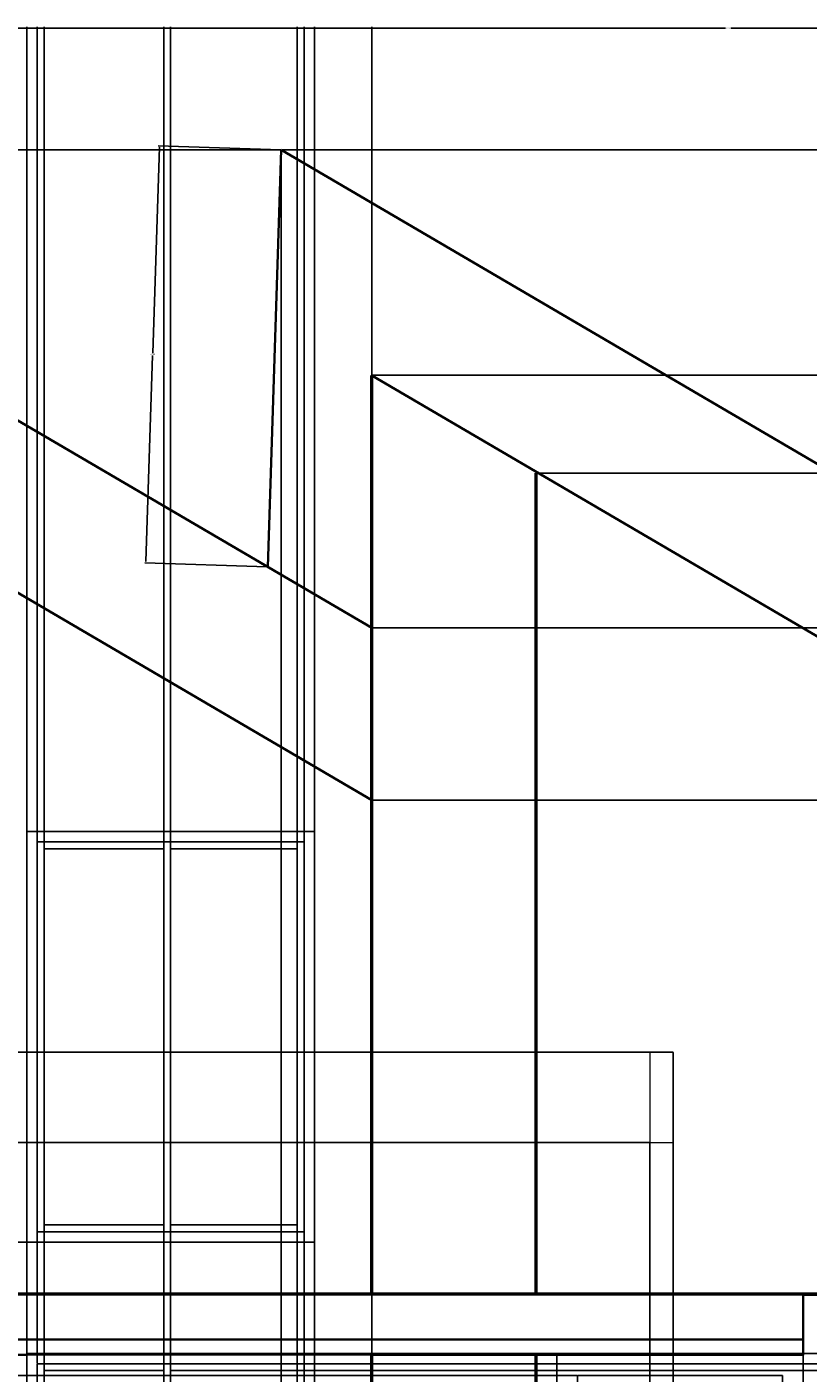
# Model space of a CAD drawing. Units: inches. Extents: x 27 to 409, y -26 to 294.
# Tile 4 of 7: x 116 to 230, y 97 to 294. Entities that reach past the tile are written whole.
import ezdxf

# ---------------------------------------------------------------- set-up
doc = ezdxf.new("R2010")
doc.units = ezdxf.units.IN
doc.header["$MEASUREMENT"] = 0
for name, color, linetype, lineweight in [('A-ANNO-DIMS', 2, 'Continuous', 18), ('A-DOOR', 3, 'Continuous', 25), ('A-ELEV', 8, 'Continuous', 18), ('A-GLAZ', 4, 'Continuous', 25), ('A-ROOF', 1, 'Continuous', 35), ('A-WALL', 7, 'Continuous', 50)]:
    doc.layers.add(name, color=color, linetype=linetype, lineweight=lineweight)
doc.styles.get("Standard").update_dxf_attribs({"font": 'arial.ttf'})
doc.dimstyles.get("Standard").update_dxf_attribs({"dimtxt": 0.18, "dimasz": 0.18, "dimexe": 0.18, "dimexo": 0.0625, "dimgap": 0.09, "dimtad": 0, "dimtih": 1, "dimtoh": 1, "dimdec": 4, "dimzin": 0, "dimdsep": 46, "dimtxsty": 'Standard', "dimcen": 0.09, "dimadec": 0, "dimazin": 0, "dimtfac": 1, "dimtdec": 4, "dimtofl": 0, "dimtmove": 0, "dimatfit": 3, "dimfxl": 1, "dimtolj": 1, "dimtzin": 0, "dimarcsym": 0})

# ---------------------------------------------------------------- blocks, each defined once
blk = doc.blocks.new('*U2')
for p, q in [((1.5, 1.5), (1.5, 58.5)), ((1.5, 58.5), (21, 58.5)), ((21, 1.5), (21, 58.5)), ((21, 58.5), (40.5, 58.5)), ((40.5, 58.5), (40.5, 1.5)), ((21, 1.5), (1.5, 1.5)), ((40.5, 1.5), (21, 1.5))]:
    blk.add_line(p, q)
blk.add_lwpolyline([(0, 0), (0, 60), (42, 60), (42, 0)], close=True)
for points in [[(20, 57.5), (20, 2.5), (2.5, 2.5), (2.5, 57.5), (20, 57.5)], [(21, 57.5), (39.5, 57.5), (39.5, 2.5), (21, 2.5)]]:
    blk.add_lwpolyline(points)
blk = doc.blocks.new('*U5')
blk.add_lwpolyline([(3.12, 0.01), (0.12, 0.01), (0.12, 84.01), (36.12, 84.01), (36.12, 0.01), (33.12, 0.01)])
for points in [[(33.12, 80.99), (33.12, 0.01), (3.12, 0.01), (3.12, 80.99)], [(29.12, 6.01), (29.12, 74.99), (7.12, 74.99), (7.12, 6.01)]]:
    blk.add_lwpolyline(points, close=True)
blk.add_circle((31.12, 42.01), 1)
blk = doc.blocks.new('*D7')
at = {"layer": 'A-ANNO-DIMS', "color": 0, "lineweight": -2, "transparency": 16777216}
for p, q in [((45.58, 108.44), (45.58, 293.63)), ((45.76, 293.45), (217.77, 293.45)), ((390.53, 293.45), (218.52, 293.45)), ((390.71, 136.32), (390.71, 293.63))]:
    blk.add_line(p, q, dxfattribs=at)
at = {"layer": 'A-ANNO-DIMS', "color": 0, "transparency": 16777216}
for points in [[(45.76, 293.48), (45.76, 293.42), (45.58, 293.45)], [(390.53, 293.48), (390.53, 293.42), (390.71, 293.45)]]:
    blk.add_solid(points, dxfattribs=at)
at = {"layer": 'Defpoints', "color": 0, "transparency": 16777216}
for p in [(390.71, 293.45), (390.71, 136.26), (45.58, 108.38)]:
    blk.add_point(p, dxfattribs=at)
at = {"layer": 'A-ANNO-DIMS', "color": 0, "transparency": 16777216, "insert": (218.14, 293.45), "char_height": 0.18, "attachment_point": 5}
blk.add_mtext('\\A1;345.1', dxfattribs=at)
blk = doc.blocks.new('*D15')
at = {"layer": 'A-ANNO-DIMS', "color": 0, "lineweight": -2, "transparency": 16777216}
for p, q in [((152.83, 275.59), (152.83, -26.5)), ((115.67, 115.93), (115.67, -26.5)), ((115.85, -26.32), (133.86, -26.32)), ((152.65, -26.32), (134.64, -26.32))]:
    blk.add_line(p, q, dxfattribs=at)
at = {"layer": 'A-ANNO-DIMS', "color": 0, "transparency": 16777216}
for points in [[(115.85, -26.29), (115.85, -26.35), (115.67, -26.32)], [(152.65, -26.29), (152.65, -26.35), (152.83, -26.32)]]:
    blk.add_solid(points, dxfattribs=at)
at = {"layer": 'Defpoints', "color": 0, "transparency": 16777216}
for p in [(152.83, 275.65), (115.67, 116), (152.83, -26.32)]:
    blk.add_point(p, dxfattribs=at)
at = {"layer": 'A-ANNO-DIMS', "color": 0, "transparency": 16777216, "insert": (134.25, -26.32), "char_height": 0.18, "attachment_point": 5}
blk.add_mtext('\\A1;37.17', dxfattribs=at)
blk = doc.blocks.new('*D16')
at = {"layer": 'A-ANNO-DIMS', "color": 0, "lineweight": -2, "transparency": 16777216}
for p, q in [((152.83, 275.59), (152.83, -26.5)), ((166.08, 180.52), (166.08, -26.5)), ((153.01, -26.32), (159, -26.32)), ((165.9, -26.32), (159.91, -26.32))]:
    blk.add_line(p, q, dxfattribs=at)
at = {"layer": 'A-ANNO-DIMS', "color": 0, "transparency": 16777216}
for points in [[(153.01, -26.29), (153.01, -26.35), (152.83, -26.32)], [(165.9, -26.29), (165.9, -26.35), (166.08, -26.32)]]:
    blk.add_solid(points, dxfattribs=at)
at = {"layer": 'Defpoints', "color": 0, "transparency": 16777216}
for p in [(152.83, 275.65), (166.08, 180.59), (166.08, -26.32)]:
    blk.add_point(p, dxfattribs=at)
at = {"layer": 'A-ANNO-DIMS', "color": 0, "transparency": 16777216, "insert": (159.45, -26.32), "char_height": 0.18, "attachment_point": 5}
blk.add_mtext('\\A1;13.242', dxfattribs=at)
blk = doc.blocks.new('*D17')
at = {"layer": 'A-ANNO-DIMS', "color": 0, "lineweight": -2, "transparency": 16777216}
for p, q in [((166.08, 180.52), (166.08, -26.5)), ((187.49, -8.58), (187.49, -26.5)), ((166.26, -26.32), (176.39, -26.32)), ((187.31, -26.32), (177.18, -26.32))]:
    blk.add_line(p, q, dxfattribs=at)
at = {"layer": 'A-ANNO-DIMS', "color": 0, "transparency": 16777216}
for points in [[(166.26, -26.29), (166.26, -26.35), (166.08, -26.32)], [(187.31, -26.29), (187.31, -26.35), (187.49, -26.32)]]:
    blk.add_solid(points, dxfattribs=at)
at = {"layer": 'Defpoints', "color": 0, "transparency": 16777216}
for p in [(166.08, 180.59), (187.49, -8.52), (187.49, -26.32)]:
    blk.add_point(p, dxfattribs=at)
at = {"layer": 'A-ANNO-DIMS', "color": 0, "transparency": 16777216, "insert": (176.78, -26.32), "char_height": 0.18, "attachment_point": 5}
blk.add_mtext('\\A1;21.42', dxfattribs=at)
blk = doc.blocks.new('*D18')
at = {"layer": 'A-ANNO-DIMS', "color": 0, "lineweight": -2, "transparency": 16777216}
for p, q in [((206.7, 130.47), (206.7, -26.5)), ((187.49, -8.58), (187.49, -26.5)), ((187.67, -26.32), (196.64, -26.32)), ((206.52, -26.32), (197.55, -26.32))]:
    blk.add_line(p, q, dxfattribs=at)
at = {"layer": 'A-ANNO-DIMS', "color": 0, "transparency": 16777216}
for points in [[(187.67, -26.29), (187.67, -26.35), (187.49, -26.32)], [(206.52, -26.29), (206.52, -26.35), (206.7, -26.32)]]:
    blk.add_solid(points, dxfattribs=at)
at = {"layer": 'Defpoints', "color": 0, "transparency": 16777216}
for p in [(206.7, 130.53), (187.49, -8.52), (206.7, -26.32)]:
    blk.add_point(p, dxfattribs=at)
at = {"layer": 'A-ANNO-DIMS', "color": 0, "transparency": 16777216, "insert": (197.09, -26.32), "char_height": 0.18, "attachment_point": 5}
blk.add_mtext('\\A1;19.203', dxfattribs=at)
blk = doc.blocks.new('*D19')
at = {"layer": 'A-ANNO-DIMS', "color": 0, "lineweight": -2, "transparency": 16777216}
for p, q in [((210.09, 143.71), (210.09, -26.5)), ((206.7, 130.47), (206.7, -26.5)), ((206.88, -26.32), (208, -26.32)), ((209.91, -26.32), (208.79, -26.32))]:
    blk.add_line(p, q, dxfattribs=at)
at = {"layer": 'A-ANNO-DIMS', "color": 0, "transparency": 16777216}
for points in [[(206.88, -26.29), (206.88, -26.35), (206.7, -26.32)], [(209.91, -26.29), (209.91, -26.35), (210.09, -26.32)]]:
    blk.add_solid(points, dxfattribs=at)
at = {"layer": 'Defpoints', "color": 0, "transparency": 16777216}
for p in [(210.09, 143.77), (206.7, 130.53), (210.09, -26.32)]:
    blk.add_point(p, dxfattribs=at)
at = {"layer": 'A-ANNO-DIMS', "color": 0, "transparency": 16777216, "insert": (208.39, -26.32), "char_height": 0.18, "attachment_point": 5}
blk.add_mtext('\\A1;3.394', dxfattribs=at)
blk = doc.blocks.new('*D20')
at = {"layer": 'A-ANNO-DIMS', "color": 0, "lineweight": -2, "transparency": 16777216}
for p, q in [((210.09, 143.71), (210.09, -26.5)), ((230.52, -8.58), (230.52, -26.5)), ((210.27, -26.32), (219.84, -26.32)), ((230.34, -26.32), (220.77, -26.32))]:
    blk.add_line(p, q, dxfattribs=at)
at = {"layer": 'A-ANNO-DIMS', "color": 0, "transparency": 16777216}
for points in [[(210.27, -26.29), (210.27, -26.35), (210.09, -26.32)], [(230.34, -26.29), (230.34, -26.35), (230.52, -26.32)]]:
    blk.add_solid(points, dxfattribs=at)
at = {"layer": 'Defpoints', "color": 0, "transparency": 16777216}
for p in [(210.09, 143.77), (230.52, -8.52), (230.52, -26.32)]:
    blk.add_point(p, dxfattribs=at)
at = {"layer": 'A-ANNO-DIMS', "color": 0, "transparency": 16777216, "insert": (220.31, -26.32), "char_height": 0.18, "attachment_point": 5}
blk.add_mtext('\\A1;20.435', dxfattribs=at)
blk = doc.blocks.new('*D30')
at = {"layer": 'A-ANNO-DIMS', "color": 0, "lineweight": -2, "transparency": 16777216}
for p, q in [((206.63, 130.53), (27.6, 130.53)), ((27.78, 130.35), (27.78, 123.45)), ((27.78, 116.18), (27.78, 123.08)), ((115.6, 116), (27.6, 116))]:
    blk.add_line(p, q, dxfattribs=at)
at = {"layer": 'A-ANNO-DIMS', "color": 0, "transparency": 16777216}
for points in [[(27.75, 130.35), (27.81, 130.35), (27.78, 130.53)], [(27.75, 116.18), (27.81, 116.18), (27.78, 116)]]:
    blk.add_solid(points, dxfattribs=at)
at = {"layer": 'Defpoints', "color": 0, "transparency": 16777216}
for p in [(27.78, 130.53), (206.7, 130.53), (115.67, 116)]:
    blk.add_point(p, dxfattribs=at)
at = {"layer": 'A-ANNO-DIMS', "color": 0, "transparency": 16777216, "insert": (27.78, 123.26), "char_height": 0.18, "attachment_point": 5}
blk.add_mtext('\\A1;14.54', dxfattribs=at)
blk = doc.blocks.new('*D31')
at = {"layer": 'A-ANNO-DIMS', "color": 0, "lineweight": -2, "transparency": 16777216}
for p, q in [((210.03, 143.77), (27.6, 143.77)), ((27.78, 143.59), (27.78, 137.34)), ((27.78, 130.71), (27.78, 136.97)), ((206.63, 130.53), (27.6, 130.53))]:
    blk.add_line(p, q, dxfattribs=at)
at = {"layer": 'A-ANNO-DIMS', "color": 0, "transparency": 16777216}
for points in [[(27.75, 143.59), (27.81, 143.59), (27.78, 143.77)], [(27.75, 130.71), (27.81, 130.71), (27.78, 130.53)]]:
    blk.add_solid(points, dxfattribs=at)
at = {"layer": 'Defpoints', "color": 0, "transparency": 16777216}
for p in [(27.78, 143.77), (210.09, 143.77), (206.7, 130.53)]:
    blk.add_point(p, dxfattribs=at)
at = {"layer": 'A-ANNO-DIMS', "color": 0, "transparency": 16777216, "insert": (27.78, 137.15), "char_height": 0.18, "attachment_point": 5}
blk.add_mtext('\\A1;13.24', dxfattribs=at)
blk = doc.blocks.new('*D32')
at = {"layer": 'A-ANNO-DIMS', "color": 0, "lineweight": -2, "transparency": 16777216}
for p, q in [((103.01, 162.94), (27.6, 162.94)), ((27.78, 162.76), (27.78, 153.54)), ((27.78, 143.95), (27.78, 153.17)), ((210.03, 143.77), (27.6, 143.77))]:
    blk.add_line(p, q, dxfattribs=at)
at = {"layer": 'A-ANNO-DIMS', "color": 0, "transparency": 16777216}
for points in [[(27.75, 162.76), (27.81, 162.76), (27.78, 162.94)], [(27.75, 143.95), (27.81, 143.95), (27.78, 143.77)]]:
    blk.add_solid(points, dxfattribs=at)
at = {"layer": 'Defpoints', "color": 0, "transparency": 16777216}
for p in [(27.78, 162.94), (103.08, 162.94), (210.09, 143.77)]:
    blk.add_point(p, dxfattribs=at)
at = {"layer": 'A-ANNO-DIMS', "color": 0, "transparency": 16777216, "insert": (27.78, 153.36), "char_height": 0.18, "attachment_point": 5}
blk.add_mtext('\\A1;19.164', dxfattribs=at)
blk = doc.blocks.new('*D38')
at = {"layer": 'A-ANNO-DIMS', "color": 0, "lineweight": -2, "transparency": 16777216}
for p, q in [((152.77, 275.65), (27.6, 275.65)), ((27.78, 275.47), (27.78, 265.88)), ((27.78, 255.93), (27.78, 265.52)), ((80.73, 255.75), (27.6, 255.75))]:
    blk.add_line(p, q, dxfattribs=at)
at = {"layer": 'A-ANNO-DIMS', "color": 0, "transparency": 16777216}
for points in [[(27.75, 275.47), (27.81, 275.47), (27.78, 275.65)], [(27.75, 255.93), (27.81, 255.93), (27.78, 255.75)]]:
    blk.add_solid(points, dxfattribs=at)
at = {"layer": 'Defpoints', "color": 0, "transparency": 16777216}
for p in [(27.78, 275.65), (152.83, 275.65), (80.8, 255.75)]:
    blk.add_point(p, dxfattribs=at)
at = {"layer": 'A-ANNO-DIMS', "color": 0, "transparency": 16777216, "insert": (27.78, 265.7), "char_height": 0.18, "attachment_point": 5}
blk.add_mtext('\\A1;19.9', dxfattribs=at)
blk = doc.blocks.new('*D44')
at = {"layer": 'A-ANNO-DIMS', "color": 0, "lineweight": -2, "transparency": 16777216}
for p, q in [((166.14, 180.59), (408.69, 180.59)), ((408.51, 180.41), (408.51, 158.6)), ((408.51, 136.44), (408.51, 158.24)), ((390.77, 136.26), (408.69, 136.26))]:
    blk.add_line(p, q, dxfattribs=at)
at = {"layer": 'A-ANNO-DIMS', "color": 0, "transparency": 16777216}
for points in [[(408.48, 180.41), (408.54, 180.41), (408.51, 180.59)], [(408.48, 136.44), (408.54, 136.44), (408.51, 136.26)]]:
    blk.add_solid(points, dxfattribs=at)
at = {"layer": 'Defpoints', "color": 0, "transparency": 16777216}
for p in [(166.08, 180.59), (408.51, 180.59), (390.71, 136.26)]:
    blk.add_point(p, dxfattribs=at)
at = {"layer": 'A-ANNO-DIMS', "color": 0, "transparency": 16777216, "insert": (408.51, 158.42), "char_height": 0.18, "attachment_point": 5}
blk.add_mtext('\\A1;44.33', dxfattribs=at)
blk = doc.blocks.new('*D45')
at = {"layer": 'A-ANNO-DIMS', "color": 0, "lineweight": -2, "transparency": 16777216}
for p, q in [((166.14, 205.78), (408.69, 205.78)), ((408.51, 205.6), (408.51, 193.36)), ((408.51, 180.77), (408.51, 193)), ((166.14, 180.59), (408.69, 180.59))]:
    blk.add_line(p, q, dxfattribs=at)
at = {"layer": 'A-ANNO-DIMS', "color": 0, "transparency": 16777216}
for points in [[(408.48, 205.6), (408.54, 205.6), (408.51, 205.78)], [(408.48, 180.77), (408.54, 180.77), (408.51, 180.59)]]:
    blk.add_solid(points, dxfattribs=at)
at = {"layer": 'Defpoints', "color": 0, "transparency": 16777216}
for p in [(166.08, 205.78), (408.51, 205.78), (166.08, 180.59)]:
    blk.add_point(p, dxfattribs=at)
at = {"layer": 'A-ANNO-DIMS', "color": 0, "transparency": 16777216, "insert": (408.51, 193.18), "char_height": 0.18, "attachment_point": 5}
blk.add_mtext('\\A1;25.194', dxfattribs=at)
blk = doc.blocks.new('*D46')
at = {"layer": 'A-ANNO-DIMS', "color": 0, "lineweight": -2, "transparency": 16777216}
for p, q in [((190.14, 228.38), (408.69, 228.38)), ((408.51, 228.2), (408.51, 217.26)), ((408.51, 205.96), (408.51, 216.9)), ((166.14, 205.78), (408.69, 205.78))]:
    blk.add_line(p, q, dxfattribs=at)
at = {"layer": 'A-ANNO-DIMS', "color": 0, "transparency": 16777216}
for points in [[(408.48, 228.2), (408.54, 228.2), (408.51, 228.38)], [(408.48, 205.96), (408.54, 205.96), (408.51, 205.78)]]:
    blk.add_solid(points, dxfattribs=at)
at = {"layer": 'Defpoints', "color": 0, "transparency": 16777216}
for p in [(190.08, 228.38), (408.51, 228.38), (166.08, 205.78)]:
    blk.add_point(p, dxfattribs=at)
at = {"layer": 'A-ANNO-DIMS', "color": 0, "transparency": 16777216, "insert": (408.51, 217.08), "char_height": 0.18, "attachment_point": 5}
blk.add_mtext('\\A1;22.6', dxfattribs=at)
blk = doc.blocks.new('*D47')
at = {"layer": 'A-ANNO-DIMS', "color": 0, "lineweight": -2, "transparency": 16777216}
for p, q in [((166.14, 242.7), (408.69, 242.7)), ((408.51, 242.52), (408.51, 235.72)), ((408.51, 228.56), (408.51, 235.36)), ((190.14, 228.38), (408.69, 228.38))]:
    blk.add_line(p, q, dxfattribs=at)
at = {"layer": 'A-ANNO-DIMS', "color": 0, "transparency": 16777216}
for points in [[(408.48, 242.52), (408.54, 242.52), (408.51, 242.7)], [(408.48, 228.56), (408.54, 228.56), (408.51, 228.38)]]:
    blk.add_solid(points, dxfattribs=at)
at = {"layer": 'Defpoints', "color": 0, "transparency": 16777216}
for p in [(166.08, 242.7), (408.51, 242.7), (190.08, 228.38)]:
    blk.add_point(p, dxfattribs=at)
at = {"layer": 'A-ANNO-DIMS', "color": 0, "transparency": 16777216, "insert": (408.51, 235.54), "char_height": 0.18, "attachment_point": 5}
blk.add_mtext('\\A1;14.318', dxfattribs=at)
blk = doc.blocks.new('*D48')
at = {"layer": 'A-ANNO-DIMS', "color": 0, "lineweight": -2, "transparency": 16777216}
for p, q in [((152.9, 275.65), (408.69, 275.65)), ((408.51, 275.47), (408.51, 259.36)), ((408.51, 242.88), (408.51, 258.99)), ((166.14, 242.7), (408.69, 242.7))]:
    blk.add_line(p, q, dxfattribs=at)
at = {"layer": 'A-ANNO-DIMS', "color": 0, "transparency": 16777216}
for points in [[(408.48, 275.47), (408.54, 275.47), (408.51, 275.65)], [(408.48, 242.88), (408.54, 242.88), (408.51, 242.7)]]:
    blk.add_solid(points, dxfattribs=at)
at = {"layer": 'Defpoints', "color": 0, "transparency": 16777216}
for p in [(152.83, 275.65), (408.51, 275.65), (166.08, 242.7)]:
    blk.add_point(p, dxfattribs=at)
at = {"layer": 'A-ANNO-DIMS', "color": 0, "transparency": 16777216, "insert": (408.51, 259.17), "char_height": 0.18, "attachment_point": 5}
blk.add_mtext('\\A1;32.954', dxfattribs=at)
blk = doc.blocks.new('*D51')
at = {"layer": 'A-ANNO-DIMS', "color": 0, "lineweight": -2, "transparency": 16777216}
for p, q in [((135.04, 276.05), (134.05, 245.94)), ((152.77, 275.65), (134.86, 276.24)), ((133.06, 215.46), (134.04, 245.58)), ((150.78, 214.71), (132.88, 215.29))]:
    blk.add_line(p, q, dxfattribs=at)
at = {"layer": 'A-ANNO-DIMS', "color": 0, "transparency": 16777216}
for points in [[(135.01, 276.05), (135.07, 276.05), (135.04, 276.23)], [(133.03, 215.46), (133.09, 215.46), (133.06, 215.28)]]:
    blk.add_solid(points, dxfattribs=at)
at = {"layer": 'Defpoints', "color": 0, "transparency": 16777216}
for p in [(135.04, 276.23), (152.83, 275.65), (150.85, 214.7)]:
    blk.add_point(p, dxfattribs=at)
at = {"layer": 'A-ANNO-DIMS', "color": 0, "transparency": 16777216, "insert": (134.05, 245.76), "char_height": 0.18, "attachment_point": 5}
blk.add_mtext('\\A1;60.98', dxfattribs=at)
blk = doc.blocks.new('*D72')
at = {"layer": 'A-ANNO-DIMS', "color": 0, "lineweight": -2, "transparency": 16777216}
for p, q in [((190.01, 99.5), (27.6, 99.5)), ((27.78, 99.32), (27.78, 98.17)), ((196.04, 96.47), (27.6, 96.47)), ((27.78, 96.65), (27.78, 97.8))]:
    blk.add_line(p, q, dxfattribs=at)
at = {"layer": 'A-ANNO-DIMS', "color": 0, "transparency": 16777216}
for points in [[(27.75, 99.32), (27.81, 99.32), (27.78, 99.5)], [(27.75, 96.65), (27.81, 96.65), (27.78, 96.47)]]:
    blk.add_solid(points, dxfattribs=at)
at = {"layer": 'Defpoints', "color": 0, "transparency": 16777216}
for p in [(27.78, 99.5), (190.08, 99.5), (196.1, 96.47)]:
    blk.add_point(p, dxfattribs=at)
at = {"layer": 'A-ANNO-DIMS', "color": 0, "transparency": 16777216, "insert": (27.78, 97.98), "char_height": 0.18, "attachment_point": 5}
blk.add_mtext('\\A1;3.023', dxfattribs=at)
blk = doc.blocks.new('*D73')
at = {"layer": 'A-ANNO-DIMS', "color": 0, "lineweight": -2, "transparency": 16777216}
for p, q in [((229.04, 101.74), (27.6, 101.74)), ((27.78, 101.56), (27.78, 100.8)), ((27.78, 99.68), (27.78, 100.44)), ((190.01, 99.5), (27.6, 99.5))]:
    blk.add_line(p, q, dxfattribs=at)
at = {"layer": 'A-ANNO-DIMS', "color": 0, "transparency": 16777216}
for points in [[(27.75, 101.56), (27.81, 101.56), (27.78, 101.74)], [(27.75, 99.68), (27.81, 99.68), (27.78, 99.5)]]:
    blk.add_solid(points, dxfattribs=at)
at = {"layer": 'Defpoints', "color": 0, "transparency": 16777216}
for p in [(27.78, 101.74), (229.1, 101.74), (190.08, 99.5)]:
    blk.add_point(p, dxfattribs=at)
at = {"layer": 'A-ANNO-DIMS', "color": 0, "transparency": 16777216, "insert": (27.78, 100.62), "char_height": 0.18, "attachment_point": 5}
blk.add_mtext('\\A1;2.24', dxfattribs=at)
blk = doc.blocks.new('*D97')
at = {"layer": 'A-ANNO-DIMS', "color": 0, "lineweight": -2, "transparency": 16777216}
for p, q in [((115.67, 99.56), (115.67, 293.63)), ((115.85, 293.45), (116.17, 293.45)), ((116.99, 293.45), (116.66, 293.45)), ((117.17, 98.27), (117.17, 293.63))]:
    blk.add_line(p, q, dxfattribs=at)
at = {"layer": 'A-ANNO-DIMS', "color": 0, "transparency": 16777216}
for points in [[(115.85, 293.48), (115.85, 293.42), (115.67, 293.45)], [(116.99, 293.48), (116.99, 293.42), (117.17, 293.45)]]:
    blk.add_solid(points, dxfattribs=at)
at = {"layer": 'Defpoints', "color": 0, "transparency": 16777216}
for p in [(117.17, 293.45), (115.67, 99.5), (117.17, 98.21)]:
    blk.add_point(p, dxfattribs=at)
at = {"layer": 'A-ANNO-DIMS', "color": 0, "transparency": 16777216, "insert": (116.42, 293.45), "char_height": 0.18, "attachment_point": 5}
blk.add_mtext('\\A1;1.5', dxfattribs=at)
blk = doc.blocks.new('*D98')
at = {"layer": 'A-ANNO-DIMS', "color": 0, "lineweight": -2, "transparency": 16777216}
for p, q in [((117.17, 98.27), (117.17, 293.63)), ((117.35, 293.45), (117.54, 293.45)), ((117.99, 293.45), (117.79, 293.45)), ((118.17, 97.27), (118.17, 293.63))]:
    blk.add_line(p, q, dxfattribs=at)
at = {"layer": 'A-ANNO-DIMS', "color": 0, "transparency": 16777216}
for points in [[(117.35, 293.48), (117.35, 293.42), (117.17, 293.45)], [(117.99, 293.48), (117.99, 293.42), (118.17, 293.45)]]:
    blk.add_solid(points, dxfattribs=at)
at = {"layer": 'Defpoints', "color": 0, "transparency": 16777216}
for p in [(118.17, 293.45), (117.17, 98.21), (118.17, 97.21)]:
    blk.add_point(p, dxfattribs=at)
at = {"layer": 'A-ANNO-DIMS', "color": 0, "transparency": 16777216, "insert": (117.67, 293.45), "char_height": 0.18, "attachment_point": 5}
blk.add_mtext('\\A1;1', dxfattribs=at)
blk = doc.blocks.new('*D99')
at = {"layer": 'A-ANNO-DIMS', "color": 0, "lineweight": -2, "transparency": 16777216}
for p, q in [((118.17, 97.27), (118.17, 293.63)), ((118.35, 293.45), (126.6, 293.45)), ((135.49, 293.45), (127.23, 293.45)), ((135.67, 97.27), (135.67, 293.63))]:
    blk.add_line(p, q, dxfattribs=at)
at = {"layer": 'A-ANNO-DIMS', "color": 0, "transparency": 16777216}
for points in [[(118.35, 293.48), (118.35, 293.42), (118.17, 293.45)], [(135.49, 293.48), (135.49, 293.42), (135.67, 293.45)]]:
    blk.add_solid(points, dxfattribs=at)
at = {"layer": 'Defpoints', "color": 0, "transparency": 16777216}
for p in [(135.67, 293.45), (118.17, 97.21), (135.67, 97.21)]:
    blk.add_point(p, dxfattribs=at)
at = {"layer": 'A-ANNO-DIMS', "color": 0, "transparency": 16777216, "insert": (126.92, 293.45), "char_height": 0.18, "attachment_point": 5}
blk.add_mtext('\\A1;17.5', dxfattribs=at)
blk = doc.blocks.new('*D100')
at = {"layer": 'A-ANNO-DIMS', "color": 0, "lineweight": -2, "transparency": 16777216}
for p, q in [((135.67, 97.27), (135.67, 293.63)), ((135.85, 293.45), (136.04, 293.45)), ((136.49, 293.45), (136.29, 293.45)), ((136.67, 98.27), (136.67, 293.63))]:
    blk.add_line(p, q, dxfattribs=at)
at = {"layer": 'A-ANNO-DIMS', "color": 0, "transparency": 16777216}
for points in [[(135.85, 293.48), (135.85, 293.42), (135.67, 293.45)], [(136.49, 293.48), (136.49, 293.42), (136.67, 293.45)]]:
    blk.add_solid(points, dxfattribs=at)
at = {"layer": 'Defpoints', "color": 0, "transparency": 16777216}
for p in [(136.67, 293.45), (135.67, 97.21), (136.67, 98.21)]:
    blk.add_point(p, dxfattribs=at)
at = {"layer": 'A-ANNO-DIMS', "color": 0, "transparency": 16777216, "insert": (136.17, 293.45), "char_height": 0.18, "attachment_point": 5}
blk.add_mtext('\\A1;1', dxfattribs=at)
blk = doc.blocks.new('*D101')
at = {"layer": 'A-ANNO-DIMS', "color": 0, "lineweight": -2, "transparency": 16777216}
for p, q in [((136.67, 98.27), (136.67, 293.63)), ((136.85, 293.45), (145.6, 293.45)), ((154.99, 293.45), (146.23, 293.45)), ((155.17, 97.27), (155.17, 293.63))]:
    blk.add_line(p, q, dxfattribs=at)
at = {"layer": 'A-ANNO-DIMS', "color": 0, "transparency": 16777216}
for points in [[(136.85, 293.48), (136.85, 293.42), (136.67, 293.45)], [(154.99, 293.48), (154.99, 293.42), (155.17, 293.45)]]:
    blk.add_solid(points, dxfattribs=at)
at = {"layer": 'Defpoints', "color": 0, "transparency": 16777216}
for p in [(155.17, 293.45), (136.67, 98.21), (155.17, 97.21)]:
    blk.add_point(p, dxfattribs=at)
at = {"layer": 'A-ANNO-DIMS', "color": 0, "transparency": 16777216, "insert": (145.92, 293.45), "char_height": 0.18, "attachment_point": 5}
blk.add_mtext('\\A1;18.5', dxfattribs=at)
blk = doc.blocks.new('*D102')
at = {"layer": 'A-ANNO-DIMS', "color": 0, "lineweight": -2, "transparency": 16777216}
for p, q in [((155.17, 97.27), (155.17, 293.63)), ((155.35, 293.45), (155.54, 293.45)), ((155.99, 293.45), (155.79, 293.45)), ((156.17, 98.27), (156.17, 293.63))]:
    blk.add_line(p, q, dxfattribs=at)
at = {"layer": 'A-ANNO-DIMS', "color": 0, "transparency": 16777216}
for points in [[(155.35, 293.48), (155.35, 293.42), (155.17, 293.45)], [(155.99, 293.48), (155.99, 293.42), (156.17, 293.45)]]:
    blk.add_solid(points, dxfattribs=at)
at = {"layer": 'Defpoints', "color": 0, "transparency": 16777216}
for p in [(156.17, 293.45), (155.17, 97.21), (156.17, 98.21)]:
    blk.add_point(p, dxfattribs=at)
at = {"layer": 'A-ANNO-DIMS', "color": 0, "transparency": 16777216, "insert": (155.67, 293.45), "char_height": 0.18, "attachment_point": 5}
blk.add_mtext('\\A1;1', dxfattribs=at)
blk = doc.blocks.new('*D103')
at = {"layer": 'A-ANNO-DIMS', "color": 0, "lineweight": -2, "transparency": 16777216}
for p, q in [((156.17, 98.27), (156.17, 293.63)), ((156.35, 293.45), (156.67, 293.45)), ((157.49, 293.45), (157.16, 293.45)), ((157.67, 99.77), (157.67, 293.63))]:
    blk.add_line(p, q, dxfattribs=at)
at = {"layer": 'A-ANNO-DIMS', "color": 0, "transparency": 16777216}
for points in [[(156.35, 293.48), (156.35, 293.42), (156.17, 293.45)], [(157.49, 293.48), (157.49, 293.42), (157.67, 293.45)]]:
    blk.add_solid(points, dxfattribs=at)
at = {"layer": 'Defpoints', "color": 0, "transparency": 16777216}
for p in [(157.67, 293.45), (157.67, 99.71), (156.17, 98.21)]:
    blk.add_point(p, dxfattribs=at)
at = {"layer": 'A-ANNO-DIMS', "color": 0, "transparency": 16777216, "insert": (156.92, 293.45), "char_height": 0.18, "attachment_point": 5}
blk.add_mtext('\\A1;1.5', dxfattribs=at)
blk = doc.blocks.new('*D104')
at = {"layer": 'A-ANNO-DIMS', "color": 0, "lineweight": -2, "transparency": 16777216}
for p, q in [((157.67, 99.77), (157.67, 293.63)), ((157.85, 293.45), (161.48, 293.45)), ((165.9, 293.45), (162.26, 293.45)), ((166.08, 99.56), (166.08, 293.63))]:
    blk.add_line(p, q, dxfattribs=at)
at = {"layer": 'A-ANNO-DIMS', "color": 0, "transparency": 16777216}
for points in [[(157.85, 293.48), (157.85, 293.42), (157.67, 293.45)], [(165.9, 293.48), (165.9, 293.42), (166.08, 293.45)]]:
    blk.add_solid(points, dxfattribs=at)
at = {"layer": 'Defpoints', "color": 0, "transparency": 16777216}
for p in [(166.08, 293.45), (157.67, 99.71), (166.08, 99.5)]:
    blk.add_point(p, dxfattribs=at)
at = {"layer": 'A-ANNO-DIMS', "color": 0, "transparency": 16777216, "insert": (161.87, 293.45), "char_height": 0.18, "attachment_point": 5}
blk.add_mtext('\\A1;8.409', dxfattribs=at)
blk = doc.blocks.new('*D110')
at = {"layer": 'A-ANNO-DIMS', "color": 0, "lineweight": -2, "transparency": 16777216}
for p, q in [((155.23, 97.21), (408.69, 97.21)), ((408.51, 97.03), (408.51, 69.89)), ((408.51, 42.39), (408.51, 69.53)), ((155.23, 42.21), (408.69, 42.21))]:
    blk.add_line(p, q, dxfattribs=at)
at = {"layer": 'A-ANNO-DIMS', "color": 0, "transparency": 16777216}
for points in [[(408.48, 97.03), (408.54, 97.03), (408.51, 97.21)], [(408.48, 42.39), (408.54, 42.39), (408.51, 42.21)]]:
    blk.add_solid(points, dxfattribs=at)
at = {"layer": 'Defpoints', "color": 0, "transparency": 16777216}
for p in [(155.17, 97.21), (408.51, 97.21), (155.17, 42.21)]:
    blk.add_point(p, dxfattribs=at)
at = {"layer": 'A-ANNO-DIMS', "color": 0, "transparency": 16777216, "insert": (408.51, 69.71), "char_height": 0.18, "attachment_point": 5}
blk.add_mtext('\\A1;55', dxfattribs=at)
blk = doc.blocks.new('*D111')
at = {"layer": 'A-ANNO-DIMS', "color": 0, "lineweight": -2, "transparency": 16777216}
for p, q in [((155.23, 97.21), (408.69, 97.21)), ((156.23, 98.21), (408.69, 98.21)), ((408.51, 98.03), (408.51, 97.89)), ((408.51, 97.39), (408.51, 97.53))]:
    blk.add_line(p, q, dxfattribs=at)
at = {"layer": 'A-ANNO-DIMS', "color": 0, "transparency": 16777216}
for points in [[(408.48, 98.03), (408.54, 98.03), (408.51, 98.21)], [(408.48, 97.39), (408.54, 97.39), (408.51, 97.21)]]:
    blk.add_solid(points, dxfattribs=at)
at = {"layer": 'Defpoints', "color": 0, "transparency": 16777216}
for p in [(155.17, 97.21), (156.17, 98.21), (408.51, 98.21)]:
    blk.add_point(p, dxfattribs=at)
at = {"layer": 'A-ANNO-DIMS', "color": 0, "transparency": 16777216, "insert": (408.51, 97.71), "char_height": 0.18, "attachment_point": 5}
blk.add_mtext('\\A1;1', dxfattribs=at)
blk = doc.blocks.new('*D112')
at = {"layer": 'A-ANNO-DIMS', "color": 0, "lineweight": -2, "transparency": 16777216}
for p, q in [((157.73, 99.71), (408.69, 99.71)), ((408.51, 99.53), (408.51, 99.14)), ((408.51, 98.39), (408.51, 98.78)), ((156.23, 98.21), (408.69, 98.21))]:
    blk.add_line(p, q, dxfattribs=at)
at = {"layer": 'A-ANNO-DIMS', "color": 0, "transparency": 16777216}
for points in [[(408.48, 99.53), (408.54, 99.53), (408.51, 99.71)], [(408.48, 98.39), (408.54, 98.39), (408.51, 98.21)]]:
    blk.add_solid(points, dxfattribs=at)
at = {"layer": 'Defpoints', "color": 0, "transparency": 16777216}
for p in [(157.67, 99.71), (408.51, 99.71), (156.17, 98.21)]:
    blk.add_point(p, dxfattribs=at)
at = {"layer": 'A-ANNO-DIMS', "color": 0, "transparency": 16777216, "insert": (408.51, 98.96), "char_height": 0.18, "attachment_point": 5}
blk.add_mtext('\\A1;1.5', dxfattribs=at)

msp = doc.modelspace()

# ---------------------------------------------------------------- linework, layer by layer
at = {"layer": 'A-ELEV'}
msp.add_lwpolyline([(206.6961, 130.5342), (210.0897, 130.5342), (210.0897, 143.7732), (206.6961, 143.7732)], close=True, dxfattribs=at)
at = {"layer": 'A-ROOF'}
for p, q in [((152.833, 275.6517), (150.8459, 214.7031)), ((45.5772, 101.7396), (229.1036, 101.7396))]:
    msp.add_line(p, q, dxfattribs=at)
for points in [[(166.0751, 242.6981), (379.7157, 117.5036), (390.7054, 136.2572), (152.833, 275.6517)], [(166.0751, 205.7788), (80.7971, 255.7521)], [(78.7499, 231.7582), (166.0751, 180.5852)], [(190.0751, 228.3803), (190.5079, 228.3803)], [(115.6666, 99.4952), (45.5772, 99.4952), (45.5772, 108.3803), (229.1036, 108.3803), (229.1036, 99.4952), (166.0751, 99.4952)]]:
    msp.add_lwpolyline(points, dxfattribs=at)
at = {"layer": 'A-WALL'}
for p, q in [((166.0751, 108.3803), (166.0751, 242.6981)), ((190.0751, 108.3803), (190.0751, 228.3803)), ((229.1036, 108.3803), (334.0751, 108.3803)), ((166.0751, 15.4825), (166.0751, 99.4952)), ((190.0751, 15.4825), (190.0751, 99.4952))]:
    msp.add_line(p, q, dxfattribs=at)
msp.add_lwpolyline([(334.0751, 144.2493), (334.0751, 108.3803), (94.0751, 108.3803)], dxfattribs=at)

# ---------------------------------------------------------------- block references
at = {"layer": 'A-DOOR'}
msp.add_blockref('*U5', (192.9798, 15.4825), dxfattribs=at)
at = {"layer": 'A-GLAZ'}
for p in [(115.6666, 115.9951), (115.6666, 39.7093)]:
    msp.add_blockref('*U2', p, dxfattribs=at)

# ---------------------------------------------------------------- dimensions: what is measured, and where the dimension line sits
at = {"layer": 'A-ANNO-DIMS'}
for base, p1, p2, override, picture, middle in [((390.7054, 293.4517), (45.5772, 108.3803), (390.7054, 136.2572), {"dimdec": 1, "dimlfac": 1, "dimrnd": 0, "dimzin": 0, "dimdsep": 46, "dimlunit": 2}, '*D7', (218.1413, 293.4517)), ((117.1666, 293.4517), (115.6666, 99.4952), (117.1666, 98.2093), {"dimdec": 1, "dimlfac": 1, "dimrnd": 0, "dimzin": 0, "dimdsep": 46, "dimlunit": 2}, '*D97', (116.4166, 293.4517)), ((118.1666, 293.4517), (117.1666, 98.2093), (118.1666, 97.2093), {"dimdec": 0, "dimlfac": 1, "dimrnd": 0, "dimzin": 0, "dimdsep": 46, "dimlunit": 2}, '*D98', (117.6666, 293.4517)), ((135.6666, 293.4517), (118.1666, 97.2093), (135.6666, 97.2093), {"dimdec": 1, "dimlfac": 1, "dimrnd": 0, "dimzin": 0, "dimdsep": 46, "dimlunit": 2}, '*D99', (126.9166, 293.4517)), ((136.6666, 293.4517), (135.6666, 97.2093), (136.6666, 98.2093), {"dimdec": 0, "dimlfac": 1, "dimrnd": 0, "dimzin": 0, "dimdsep": 46, "dimlunit": 2}, '*D100', (136.1666, 293.4517)), ((155.1666, 293.4517), (136.6666, 98.2093), (155.1666, 97.2093), {"dimdec": 1, "dimlfac": 1, "dimrnd": 0, "dimzin": 0, "dimdsep": 46, "dimlunit": 2}, '*D101', (145.9166, 293.4517)), ((156.1666, 293.4517), (155.1666, 97.2093), (156.1666, 98.2093), {"dimdec": 0, "dimlfac": 1, "dimrnd": 0, "dimzin": 0, "dimdsep": 46, "dimlunit": 2}, '*D102', (155.6666, 293.4517)), ((157.6666, 293.4517), (156.1666, 98.2093), (157.6666, 99.7093), {"dimdec": 1, "dimlfac": 1, "dimrnd": 0, "dimzin": 0, "dimdsep": 46, "dimlunit": 2}, '*D103', (156.9166, 293.4517)), ((166.07506, 293.45166), (157.66655, 99.70931), (166.07506, 99.49521), {"dimdec": 3, "dimlfac": 1, "dimrnd": 0, "dimzin": 0, "dimdsep": 46, "dimlunit": 2}, '*D104', (161.8708, 293.45166)), ((152.833, -26.3175), (115.6666, 115.9951), (152.833, 275.6517), {"dimdec": 2, "dimlfac": 1, "dimrnd": 0, "dimzin": 0, "dimdsep": 46, "dimlunit": 2}, '*D15', (134.2498, -26.3175)), ((166.0751, -26.3175), (152.833, 275.6517), (166.0751, 180.5852), {"dimdec": 3, "dimlfac": 1, "dimrnd": 0, "dimzin": 0, "dimdsep": 46, "dimlunit": 2}, '*D16', (159.454, -26.3175)), ((187.493, -26.3175), (166.0751, 180.5852), (187.493, -8.5175), {"dimdec": 2, "dimlfac": 1, "dimrnd": 0, "dimzin": 0, "dimdsep": 46, "dimlunit": 2}, '*D17', (176.784, -26.3175)), ((210.0897, -26.3175), (206.6961, 130.5342), (210.0897, 143.7732), {"dimdec": 3, "dimlfac": 1, "dimrnd": 0, "dimzin": 0, "dimdsep": 46, "dimlunit": 2}, '*D19', (208.3929, -26.3175)), ((230.5245, -26.3175), (210.0897, 143.7732), (230.5245, -8.5175), {"dimdec": 3, "dimlfac": 1, "dimrnd": 0, "dimzin": 0, "dimdsep": 46, "dimlunit": 2}, '*D20', (220.3071, -26.3175)), ((206.6961, -26.3175), (187.493, -8.5175), (206.6961, 130.5342), {"dimdec": 3, "dimlfac": 1, "dimrnd": 0, "dimzin": 0, "dimdsep": 46, "dimlunit": 2}, '*D18', (197.0945, -26.3175))]:
    dim = msp.add_linear_dim(base=base, p1=p1, p2=p2, dimstyle='Standard', override=override, dxfattribs=at)
    dim.commit()
    dim.dimension.update_dxf_attribs({"geometry": picture, "text_midpoint": middle})
for base, p1, p2, angle, override, picture, middle in [((27.7772, 275.6517), (80.7971, 255.7521), (152.833, 275.6517), 90, {"dimdec": 1, "dimlfac": 1, "dimrnd": 0, "dimzin": 0, "dimdsep": 46, "dimlunit": 2}, '*D38', (27.7772, 265.7019)), ((135.0424, 276.2317), (150.8459, 214.7031), (152.833, 275.6517), 88.132695, {"dimdec": 2, "dimlfac": 1, "dimrnd": 0, "dimzin": 0, "dimdsep": 46, "dimlunit": 2}, '*D51', (134.0489, 245.7574)), ((408.5054, 275.6517), (166.0751, 242.6981), (152.833, 275.6517), 90, {"dimdec": 3, "dimlfac": 1, "dimrnd": 0, "dimzin": 0, "dimdsep": 46, "dimlunit": 2}, '*D48', (408.5054, 259.1749)), ((408.5054, 242.6981), (190.0751, 228.3803), (166.0751, 242.6981), 90, {"dimdec": 3, "dimlfac": 1, "dimrnd": 0, "dimzin": 0, "dimdsep": 46, "dimlunit": 2}, '*D47', (408.5054, 235.5392)), ((408.5054, 228.3803), (166.0751, 205.7788), (190.0751, 228.3803), 90, {"dimdec": 1, "dimlfac": 1, "dimrnd": 0, "dimzin": 0, "dimdsep": 46, "dimlunit": 2}, '*D46', (408.5054, 217.0795)), ((408.5054, 205.7788), (166.0751, 180.5852), (166.0751, 205.7788), 90, {"dimdec": 3, "dimlfac": 1, "dimrnd": 0, "dimzin": 0, "dimdsep": 46, "dimlunit": 2}, '*D45', (408.5054, 193.182)), ((408.5054, 180.5852), (390.7054, 136.2572), (166.0751, 180.5852), 90, {"dimdec": 2, "dimlfac": 1, "dimrnd": 0, "dimzin": 0, "dimdsep": 46, "dimlunit": 2}, '*D44', (408.5054, 158.4212)), ((27.7772, 162.937), (210.0897, 143.7732), (103.0751, 162.937), 90, {"dimdec": 3, "dimlfac": 1, "dimrnd": 0, "dimzin": 0, "dimdsep": 46, "dimlunit": 2}, '*D32', (27.7772, 153.3551)), ((27.7772, 143.7732), (206.6961, 130.5342), (210.0897, 143.7732), 90, {"dimdec": 2, "dimlfac": 1, "dimrnd": 0, "dimzin": 0, "dimdsep": 46, "dimlunit": 2}, '*D31', (27.7772, 137.1537)), ((27.7772, 130.5342), (115.6666, 115.9951), (206.6961, 130.5342), 90, {"dimdec": 2, "dimlfac": 1, "dimrnd": 0, "dimzin": 0, "dimdsep": 46, "dimlunit": 2}, '*D30', (27.7772, 123.2647)), ((27.7772, 101.7396), (190.0751, 99.4952), (229.1036, 101.7396), 90, {"dimdec": 2, "dimlfac": 1, "dimrnd": 0, "dimzin": 0, "dimdsep": 46, "dimlunit": 2}, '*D73', (27.7772, 100.6174)), ((27.7772, 99.4952), (196.1036, 96.4722), (190.0751, 99.4952), 90, {"dimdec": 3, "dimlfac": 1, "dimrnd": 0, "dimzin": 0, "dimdsep": 46, "dimlunit": 2}, '*D72', (27.7772, 97.9837)), ((408.5054, 99.7093), (156.1666, 98.2093), (157.6666, 99.7093), 90, {"dimdec": 1, "dimlfac": 1, "dimrnd": 0, "dimzin": 0, "dimdsep": 46, "dimlunit": 2}, '*D112', (408.5054, 98.9593)), ((408.5054, 98.2093), (155.1666, 97.2093), (156.1666, 98.2093), 90, {"dimdec": 0, "dimlfac": 1, "dimrnd": 0, "dimzin": 0, "dimdsep": 46, "dimlunit": 2}, '*D111', (408.5054, 97.7093)), ((408.5054, 97.2093), (155.1666, 42.2093), (155.1666, 97.2093), 90, {"dimdec": 0, "dimlfac": 1, "dimrnd": 0, "dimzin": 0, "dimdsep": 46, "dimlunit": 2}, '*D110', (408.5054, 69.7093))]:
    dim = msp.add_linear_dim(base=base, p1=p1, p2=p2, angle=angle, dimstyle='Standard', override=override, dxfattribs=at)
    dim.commit()
    dim.dimension.update_dxf_attribs({"geometry": picture, "text_midpoint": middle})

doc.saveas('drawing.dxf')
